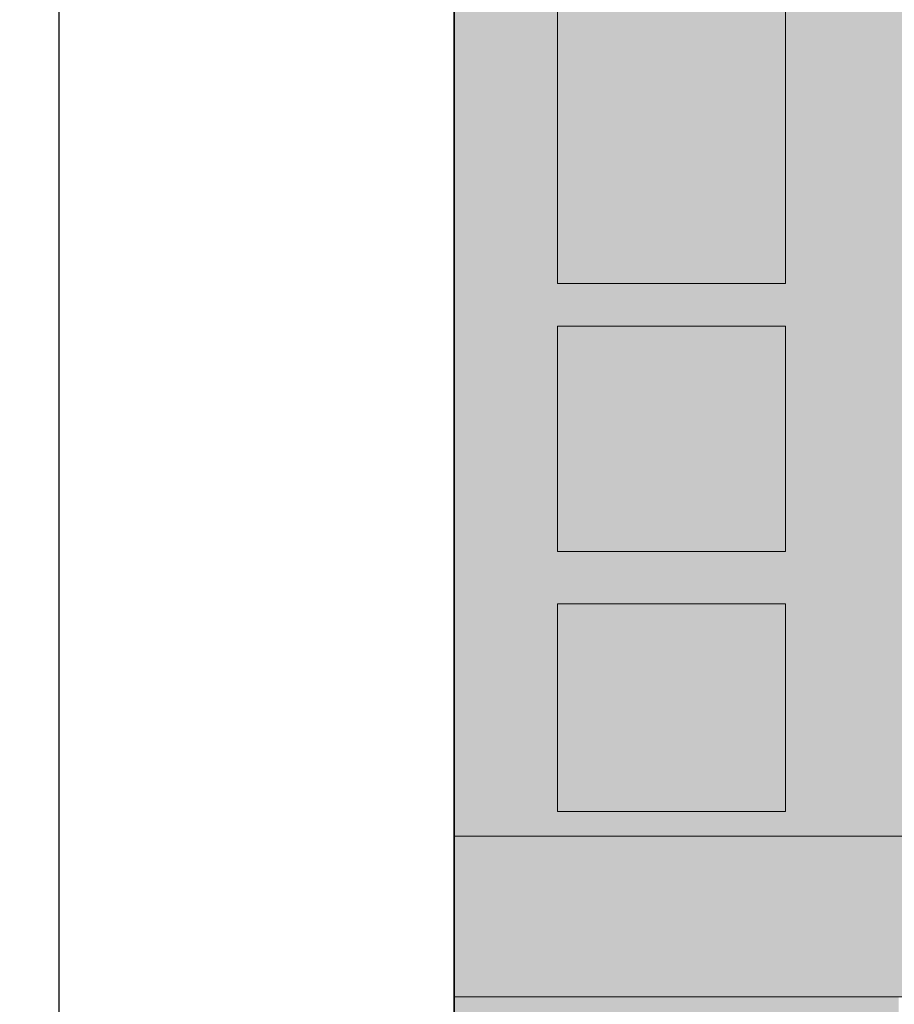
# Model space of a CAD drawing. Units: inches. Extents: x 1704 to 6393, y -157 to 1172.
# Tile 18 of 122: x 1823 to 1975, y 201 to 372. Entities that reach past the tile are written whole.
import ezdxf

# ---------------------------------------------------------------- set-up
doc = ezdxf.new("R2010")
doc.units = ezdxf.units.IN
doc.header["$MEASUREMENT"] = 0
for name, color, linetype, lineweight in [('A-ANNO-DIMS', 7, 'Continuous', 13), ('C-PROP', 7, 'Continuous', 35), ('L-HRDS', 8, 'Continuous', 18)]:
    doc.layers.add(name, color=color, linetype=linetype, lineweight=lineweight)
doc.layers.add('L-HRDS-PATT', color=9, linetype='Continuous', lineweight=13, true_color=0xc5c1ba)
doc.layers.add('L-PLNT-PATT', color=253, linetype='Continuous', lineweight=13, true_color=0x9abc8f)
doc.styles.get("Standard").update_dxf_attribs({"font": 'arial.ttf'})
doc.dimstyles.get("Standard").update_dxf_attribs({"dimtxt": 6, "dimasz": 2, "dimexe": 0.18, "dimexo": 0.0625, "dimgap": 0.09, "dimtad": 0, "dimtih": 1, "dimtoh": 1, "dimdec": 1, "dimzin": 0, "dimdsep": 46, "dimlunit": 3, "dimtxsty": 'Standard', "dimblk": 'ARCHTICK', "dimcen": 0.09, "dimadec": 0, "dimazin": 0, "dimtfac": 1, "dimtdec": 1, "dimtofl": 0, "dimtmove": 0, "dimatfit": 3, "dimfxl": 1, "dimtolj": 1, "dimtzin": 0, "dimarcsym": 0})

# ---------------------------------------------------------------- blocks, each defined once
blk = doc.blocks.new('_ArchTick')
at = {"color": 0, "linetype": 'ByBlock', "const_width": 0.15}
blk.add_lwpolyline([(-0.5, -0.5), (0.5, 0.5)], dxfattribs=at)
blk = doc.blocks.new('*D93')
at = {"layer": 'A-ANNO-DIMS', "color": 0, "lineweight": -2, "transparency": 16777216}
for p, q in [((2605.29, 895.21), (1829.7, 895.21)), ((1829.88, 895.21), (1829.88, 495.87)), ((1829.88, 90.21), (1829.88, 489.56)), ((2605.29, 90.21), (1829.7, 90.21))]:
    blk.add_line(p, q, dxfattribs=at)
at = {"layer": 'Defpoints', "color": 0, "lineweight": -3, "transparency": 16777216}
for p in [(2605.35, 895.21), (1829.88, 90.21), (2605.35, 90.21)]:
    blk.add_point(p, dxfattribs=at)
at = {"layer": 'A-ANNO-DIMS', "color": 0, "lineweight": -2, "transparency": 16777216, "xscale": 2, "yscale": 2, "zscale": 2}
for p, rotation in [((1829.88, 895.21), 90), ((1829.88, 90.21), 270)]:
    blk.add_blockref('_ArchTick', p, dxfattribs=dict(at, rotation=rotation))
at = {"layer": 'A-ANNO-DIMS', "color": 0, "transparency": 16777216, "insert": (1829.88, 492.71), "char_height": 6, "attachment_point": 5}
blk.add_mtext('\\A1;805', dxfattribs=at)

msp = doc.modelspace()

# ---------------------------------------------------------------- hatches: boundary and pattern name
at = {"layer": 'L-HRDS-PATT', "transparency": 33554643}
h = msp.add_hatch(color=256, dxfattribs=at)
h.dxf.hatch_style = 1
h.paths.add_polyline_path([(1955.732, 380.213), (1916.214, 380.213), (1916.214, 325.779), (1955.732, 325.779)])
h.paths.add_polyline_path([(1955.732, 318.405), (1916.214, 318.405), (1916.214, 279.355), (1955.732, 279.355)])
h.paths.add_polyline_path([(1955.732, 270.314), (1916.214, 270.314), (1916.214, 234.313), (1955.732, 234.313)])
h.paths.add_polyline_path([(2073.349, 230.029), (1898.349, 230.029), (1898.349, 202.213), (2073.349, 202.213)])
at = {"layer": 'L-PLNT-PATT', "transparency": 33554643}
h = msp.add_hatch(color=256, dxfattribs=at)
h.dxf.hatch_style = 1
h.paths.add_polyline_path([(2073.349, 364.213), (2029.19, 364.213), (2029.19, 372.213), (2073.349, 372.213), (2073.349, 380.213), (1955.732, 380.213), (1955.732, 325.779), (1916.214, 325.779), (1916.214, 380.213), (1898.349, 380.213), (1898.349, 230.029), (2073.349, 230.029)])
h.paths.add_polyline_path([(1955.732, 279.355), (1916.214, 279.355), (1916.214, 318.405), (1955.732, 318.405)], flags=16)
h.paths.add_polyline_path([(1955.732, 270.314), (1955.732, 234.313), (1916.214, 234.313), (1916.214, 270.314)], flags=16)
h = msp.add_hatch(color=256, dxfattribs=at)
h.dxf.hatch_style = 1
h.paths.add_polyline_path([(1975.349, 202.213), (1898.349, 202.213), (1898.349, -3.787), (1975.349, -3.787)])

# ---------------------------------------------------------------- linework, layer by layer
at = {"layer": 'C-PROP'}
msp.add_line((1898.349, -3.787), (1898.349, 1033.213), dxfattribs=at)
at = {"layer": 'L-HRDS'}
msp.add_line((1975.349, 202.213), (1898.349, 202.213), dxfattribs=at)
for points in [[(1916.214, 380.213), (1955.732, 380.213), (1955.732, 325.779), (1916.214, 325.779)], [(1916.214, 318.405), (1955.732, 318.405), (1955.732, 279.355), (1916.214, 279.355)], [(1916.214, 270.314), (1955.732, 270.314), (1955.732, 234.313), (1916.214, 234.313)], [(1898.349, 202.213), (2073.349, 202.213), (2073.349, 230.029), (1898.349, 230.029)]]:
    msp.add_lwpolyline(points, close=True, dxfattribs=at)

# ---------------------------------------------------------------- dimensions: what is measured, and where the dimension line sits
at = {"layer": 'A-ANNO-DIMS'}
dim = msp.add_linear_dim(base=(1829.878, 90.213), p1=(2605.349, 895.213), p2=(2605.349, 90.213), angle=90, dimstyle='Standard', override={"dimdec": 0, "dimlfac": 1, "dimrnd": 0, "dimzin": 0, "dimdsep": 46, "dimlunit": 2}, dxfattribs=at)
dim.commit()
dim.dimension.update_dxf_attribs({"geometry": '*D93', "text_midpoint": (1829.878, 492.713)})

doc.saveas('drawing.dxf')
